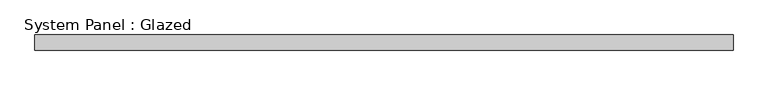
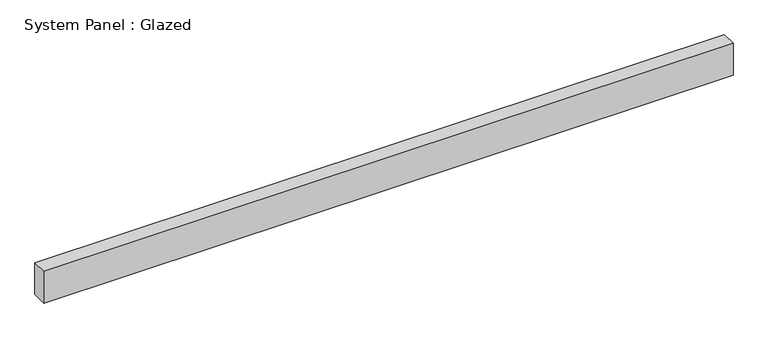
"""IFC4 building model written with IfcOpenShell, lengths in millimetres: plate geometry, System Panel : Glazed."""

from ifc_helpers import new_model, si_unit, origin, origin_with_axes, place, context, project, spatial, polyline, outline, extrude, source, transform, mapped, element, save


def system_panel_glazed_8661f242(model_context):
    return source(origin(), model_context, "Body", "SweptSolid", [
        extrude(outline(polyline([(587.3750001, 19.05), (-587.3750001, 19.05), (-587.3750001, 44.45), (587.3750001, 44.45), (587.3750001, 19.05)])), origin_with_axes(), (0.0, 0.0, 1.0), 57.15),
    ])


if __name__ == "__main__":
    model = new_model("IFC4")
    model_context = context("Model", 3, world=origin())
    ifc_project = project(units=[si_unit("LENGTHUNIT", "METRE", prefix="MILLI")], contexts=[model_context])
    site = spatial("IfcSite", under=ifc_project)
    building = spatial("IfcBuilding", under=site)
    placement = place(None, origin())
    system_panel_glazed_shape = system_panel_glazed_8661f242(model_context)
    element("IfcPlate", 1, ObjectType="System Panel : Glazed", at=placement, inside=building, context=model_context, shape_type="MappedRepresentation", body=[
        mapped(system_panel_glazed_shape, transform((0.0, 0.0, 0.0), x_axis=(1.0, 0.0, 0.0), y_axis=(0.0, 1.0, 0.0), z_axis=(0.0, 0.0, 1.0))),
    ])
    save(model, "model.ifc")

# Revit data of these elements
# Type "System Panel : Glazed"
#   Construction Type Id = "GSP4R"
#   Analytic Construction = "1/8 in Pilkington single glazing"
#   Visual Light Transmittance = 0.9
#   Solar Heat Gain Coefficient = 0.86
#   Heat Transfer Coefficient (U) = 1.18115 BTU/(h·ft²·°F)
#   Define Thermal Properties by = 1
# Element 1 (IfcPlate, "System Panel : Glazed")
#   Materials on its faces: "Glass"
# Materials
#   "Glass": class "Glass", colour RGB 0 128 192, transparency 0.75, Description = "Soda Lime Glass", Cost = 0
